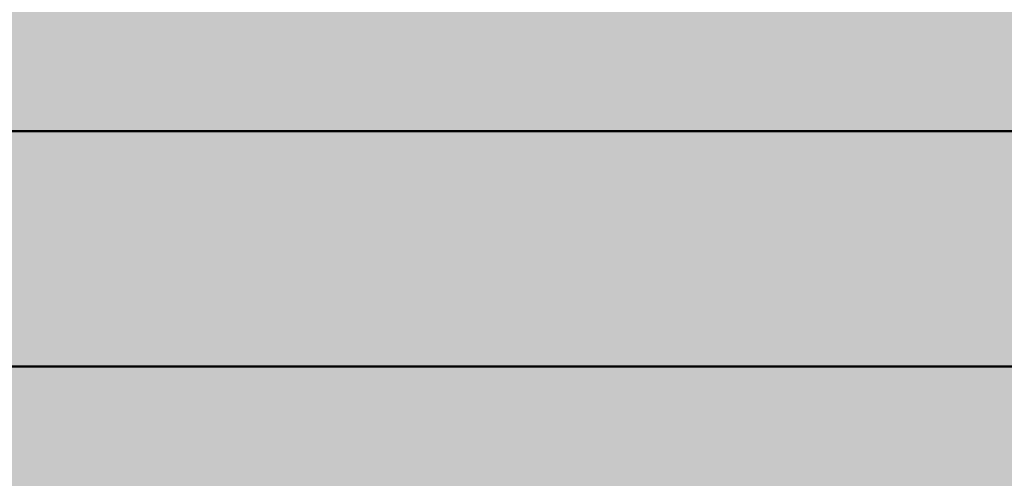
# Model space of a CAD drawing. Units: millimetres. Extents: x 0 to 2267, y 0 to 1823.
# Tile 138 of 256: x 1760 to 1802, y 1113 to 1132. Entities that reach past the tile are written whole.
import ezdxf

# ---------------------------------------------------------------- set-up
doc = ezdxf.new("R2010")
doc.units = ezdxf.units.MM
doc.header["$MEASUREMENT"] = 0
for name, color, linetype, lineweight in [('M-DIMS', 2, 'Continuous', 25), ('M-HATC', 252, 'Continuous', 18), ('M-OUTL', 7, 'Continuous', 50)]:
    doc.layers.add(name, color=color, linetype=linetype, lineweight=lineweight)
doc.styles.get("Standard").update_dxf_attribs({"font": 'arial.ttf'})
doc.dimstyles.get("Standard").update_dxf_attribs({"dimtxt": 7, "dimasz": 4, "dimexe": 0.18, "dimexo": 0.0625, "dimgap": 0.09, "dimtad": 0, "dimdec": 0, "dimzin": 0, "dimdsep": 46, "dimtxsty": 'Standard', "dimcen": 0.09, "dimadec": 0, "dimazin": 0, "dimtfac": 1, "dimtdec": 0, "dimtofl": 0, "dimtmove": 0, "dimatfit": 3, "dimfxl": 1, "dimtolj": 1, "dimtzin": 0, "dimarcsym": 0})

# ---------------------------------------------------------------- blocks, each defined once
blk = doc.blocks.new('*D1')
at = {"layer": 'Defpoints', "color": 0, "transparency": 16777216}
for p in [(1593.429, 1127.417), (1843.429, 1127.417), (1843.429, 955.628)]:
    blk.add_point(p, dxfattribs=at)
at = {"layer": 'M-DIMS', "color": 0, "lineweight": -2, "transparency": 16777216}
for p, q in [((1593.429, 1127.355), (1593.429, 955.448)), ((1843.429, 1127.355), (1843.429, 955.448)), ((1597.429, 955.628), (1710.558, 955.628)), ((1839.429, 955.628), (1726.3, 955.628))]:
    blk.add_line(p, q, dxfattribs=at)
at = {"layer": 'M-DIMS', "color": 0, "transparency": 16777216}
for points in [[(1597.429, 956.294), (1597.429, 954.961), (1593.429, 955.628)], [(1839.429, 956.294), (1839.429, 954.961), (1843.429, 955.628)]]:
    blk.add_solid(points, dxfattribs=at)
at = {"layer": 'M-DIMS', "color": 0, "transparency": 16777216, "insert": (1718.429, 955.628), "char_height": 7, "attachment_point": 5}
blk.add_mtext('\\A1;250', dxfattribs=at)

msp = doc.modelspace()

# ---------------------------------------------------------------- hatches: boundary and pattern name
at = {"layer": 'M-HATC'}
h = msp.add_hatch(color=256, dxfattribs=at)
h.dxf.hatch_style = 1
h.paths.add_polyline_path([(2065.771, 1618.062, 0.236068), (2055.771, 1638.062), (1381.087, 1638.062, 0.236068), (1371.087, 1618.062), (1371.087, 1603.062), (2055.771, 1603.062), (2065.771, 1603.062)])
h.paths.add_polyline_path([(2062.772, 1550.296), (2062.772, 1560.296), (1374.086, 1560.296), (1374.086, 1550.296), (1374.086, 1540.296), (1384.086, 1540.296), (1389.086, 1540.296), (2062.772, 1540.296)])
h.paths.add_polyline_path([(1930.929, 1282.766), (1505.929, 1282.766), (1587.628, 1235.597, 0.131652), (1600.128, 1232.247), (1836.73, 1232.247, 0.131652), (1849.23, 1235.597)])
h.paths.add_polyline_path([(1930.929, 1117.417), (1905.929, 1117.417), (1505.929, 1117.417), (1505.929, 1077.417), (1930.929, 1077.417)])
h = msp.add_hatch(color=256, dxfattribs=at)
h.dxf.hatch_style = 1
h.paths.add_polyline_path([(2055.771, 1603.062), (1381.087, 1603.062), (1381.087, 1598.062), (2055.771, 1598.062)])
h.paths.add_polyline_path([(2055.771, 1598.062), (1381.087, 1598.062), (1381.087, 1593.062), (2055.771, 1593.062)])
h.paths.add_polyline_path([(2051.307, 1536.761), (1385.55, 1536.761), (1385.55, 1526.761), (1387.55, 1526.761), (1388.537, 1525.053), (1385.332, 1521.233), (1385.332, 1521.223), (2050.254, 1522.749), (2048.321, 1525.053), (2049.307, 1526.761), (2051.307, 1526.761)])
edge = h.paths.add_edge_path()
edge.add_arc((1847.535, 1379.149), 135, 222.60306, 222.89085, ccw=False)
edge.add_line((1748.166, 1287.766), (1683.092, 1287.766))
edge.add_arc((1583.724, 1379.149), 135, 317.10915, 317.39694, ccw=False)
edge.add_arc((1678.969, 1290.671), 5, 222.8909, 317.1091, ccw=False)
edge.add_arc((1774.213, 1379.149), 135, 222.60306, 222.89085, ccw=False)
edge.add_line((1674.845, 1287.766), (1609.771, 1287.766))
edge.add_arc((1510.403, 1379.149), 135, 317.10915, 317.39694, ccw=False)
edge.add_arc((1605.647, 1290.671), 5, 222.8909, 317.1091, ccw=False)
edge.add_arc((1700.892, 1379.149), 135, 222.60306, 222.89085, ccw=False)
edge.add_line((1601.524, 1287.766), (1536.45, 1287.766))
edge.add_arc((1437.081, 1379.149), 135, 317.10915, 317.39694, ccw=False)
edge.add_arc((1532.326, 1290.671), 5, 222.8909, 317.1091, ccw=False)
edge.add_arc((1627.571, 1379.149), 135, 222.60306, 222.89085, ccw=False)
edge.add_line((1528.203, 1287.766), (1505.929, 1287.766))
edge.add_spline(control_points=[(1505.929, 1287.766), (1504.262, 1287.766), (1504.262, 1282.766), (1505.929, 1282.766)], knot_values=[0, 0, 0, 0, 5, 5, 5, 5], degree=3, periodic=0)
edge.add_line((1505.929, 1282.766), (1930.929, 1282.766))
edge.add_spline(control_points=[(1930.929, 1282.766), (1932.596, 1282.766), (1932.596, 1287.766), (1930.929, 1287.766)], knot_values=[0, 0, 0, 0, 5, 5, 5, 5], degree=3, periodic=0)
edge.add_line((1930.929, 1287.766), (1903.056, 1287.766))
edge.add_arc((1803.688, 1379.149), 135, 317.10915, 317.39694, ccw=False)
edge.add_arc((1898.932, 1290.671), 5, 222.8909, 317.1091, ccw=False)
edge.add_arc((1994.177, 1379.149), 135, 222.60306, 222.89085, ccw=False)
edge.add_line((1894.809, 1287.766), (1829.735, 1287.766))
edge.add_arc((1730.366, 1379.149), 135, 317.10915, 317.39694, ccw=False)
edge.add_arc((1825.611, 1290.671), 5, 222.8909, 317.1091, ccw=False)
edge.add_arc((1920.856, 1379.149), 135, 222.60306, 222.89085, ccw=False)
edge.add_line((1821.487, 1287.766), (1756.413, 1287.766))
edge.add_arc((1657.045, 1379.149), 135, 317.10915, 317.39694, ccw=False)
edge.add_arc((1752.29, 1290.671), 5, 222.8909, 317.1091, ccw=False)
edge = h.paths.add_edge_path()
edge.add_spline(control_points=[(1843.429, 1227.247), (1845.096, 1227.247), (1845.096, 1232.247), (1843.429, 1232.247)], knot_values=[0, 0, 0, 0, 5, 5, 5, 5], degree=3, periodic=0)
edge.add_line((1843.429, 1232.247), (1593.429, 1232.247))
edge.add_spline(control_points=[(1593.429, 1232.247), (1591.762, 1232.247), (1591.762, 1227.247), (1593.429, 1227.247)], knot_values=[0, 0, 0, 0, 5, 5, 5, 5], degree=3, periodic=0)
edge.add_line((1593.429, 1227.247), (1843.429, 1227.247))
h.paths.add_polyline_path([(1905.929, 1127.417), (1530.929, 1127.417, 0.414214), (1520.929, 1117.417), (1530.929, 1117.417), (1915.929, 1117.417, 0.414214)])
edge = h.paths.add_edge_path()
edge.add_arc((1397.086, 1498.408), 12.73, 90.7821, 190.8787, ccw=False)
edge.add_line((1396.912, 1511.136), (1428.01, 1511.349))
edge.add_line((1428.01, 1511.349), (1433.01, 1511.349))
edge.add_line((1433.01, 1511.349), (1434.439, 1511.349))
edge.add_arc((1419.474, 1498.08), 20, 41.561, 74.0821)
edge.add_line((1424.959, 1517.314), (1399.935, 1517.256))
edge.add_spline(control_points=[(1399.931, 1517.256), (1399.884, 1517.213), (1399.833, 1517.169), (1399.777, 1517.124)], knot_values=[11.567499, 11.567499, 11.567499, 11.567499, 11.814249, 11.814249, 11.814249, 11.814249], degree=3, periodic=0)
edge.add_spline(control_points=[(1399.633, 1517.01), (1399.583, 1516.972), (1399.531, 1516.934), (1399.476, 1516.895)], knot_values=[11.167718, 11.167718, 11.167718, 11.167718, 11.365188, 11.365188, 11.365188, 11.365188], degree=3, periodic=0)
edge.add_spline(control_points=[(1399.34, 1516.8), (1399.151, 1516.672), (1398.938, 1516.538), (1398.704, 1516.399)], knot_values=[10.376405, 10.376405, 10.376405, 10.376405, 11.00994, 11.00994, 11.00994, 11.00994], degree=3, periodic=0)
edge.add_spline(control_points=[(1398.657, 1516.372), (1398.579, 1516.326), (1398.498, 1516.28), (1398.415, 1516.233)], knot_values=[10.125175, 10.125175, 10.125175, 10.125175, 10.334406, 10.334406, 10.334406, 10.334406], degree=3, periodic=0)
edge.add_spline(control_points=[(1398.264, 1516.149), (1398.196, 1516.111), (1398.126, 1516.073), (1398.055, 1516.035)], knot_values=[9.832246, 9.832246, 9.832246, 9.832246, 9.999658, 9.999658, 9.999658, 9.999658], degree=3, periodic=0)
edge.add_spline(control_points=[(1397.999, 1516.005), (1397.731, 1515.862), (1397.446, 1515.717), (1397.147, 1515.571)], knot_values=[9.161808, 9.161808, 9.161808, 9.161808, 9.787769, 9.787769, 9.787769, 9.787769], degree=3, periodic=0)
edge.add_spline(control_points=[(1397.147, 1515.571), (1396.842, 1515.423), (1396.522, 1515.274), (1396.191, 1515.126)], knot_values=[8.524455, 8.524455, 8.524455, 8.524455, 9.161808, 9.161808, 9.161808, 9.161808], degree=3, periodic=0)
edge.add_spline(control_points=[(1396.078, 1515.076), (1395.985, 1515.035), (1395.892, 1514.994), (1395.798, 1514.953)], knot_values=[8.275193, 8.275193, 8.275193, 8.275193, 8.451726, 8.451726, 8.451726, 8.451726], degree=3, periodic=0)
edge.add_spline(control_points=[(1395.602, 1514.869), (1395.5, 1514.826), (1395.397, 1514.782), (1395.293, 1514.739)], knot_values=[7.962917, 7.962917, 7.962917, 7.962917, 8.152764, 8.152764, 8.152764, 8.152764], degree=3, periodic=0)
edge.add_spline(control_points=[(1395.212, 1514.706), (1394.828, 1514.547), (1394.435, 1514.393), (1394.036, 1514.244)], knot_values=[7.21254, 7.21254, 7.21254, 7.21254, 7.913148, 7.913148, 7.913148, 7.913148], degree=3, periodic=0)
edge.add_spline(control_points=[(1394.036, 1514.244), (1393.708, 1514.121), (1393.375, 1514.003), (1393.043, 1513.889)], knot_values=[6.633733, 6.633733, 6.633733, 6.633733, 7.21254, 7.21254, 7.21254, 7.21254], degree=3, periodic=0)
edge.add_spline(control_points=[(1392.821, 1513.815), (1392.72, 1513.781), (1392.618, 1513.748), (1392.517, 1513.715)], knot_values=[6.328796, 6.328796, 6.328796, 6.328796, 6.505493, 6.505493, 6.505493, 6.505493], degree=3, periodic=0)
edge.add_spline(control_points=[(1392.517, 1513.715), (1392.319, 1513.652), (1392.121, 1513.59), (1391.924, 1513.531)], knot_values=[5.984605, 5.984605, 5.984605, 5.984605, 6.328796, 6.328796, 6.328796, 6.328796], degree=3, periodic=0)
edge.add_spline(control_points=[(1391.792, 1513.491), (1391.312, 1513.35), (1390.838, 1513.224), (1390.378, 1513.117)], knot_values=[5.066697, 5.066697, 5.066697, 5.066697, 5.907055, 5.907055, 5.907055, 5.907055], degree=3, periodic=0)
edge.add_spline(control_points=[(1390.378, 1513.117), (1390.18, 1513.071), (1389.984, 1513.028), (1389.791, 1512.99)], knot_values=[4.70367, 4.70367, 4.70367, 4.70367, 5.066695, 5.066695, 5.066695, 5.066695], degree=3, periodic=0)
edge.add_spline(control_points=[(1389.422, 1512.92), (1389.246, 1512.889), (1389.073, 1512.862), (1388.904, 1512.838)], knot_values=[4.130571, 4.130571, 4.130571, 4.130571, 4.469816, 4.469816, 4.469816, 4.469816], degree=3, periodic=0)
edge.add_spline(control_points=[(1388.904, 1512.838), (1388.591, 1512.795), (1388.291, 1512.764), (1388.007, 1512.749)], knot_values=[3.504031, 3.504031, 3.504031, 3.504031, 4.130571, 4.130571, 4.130571, 4.130571], degree=3, periodic=0)
edge.add_spline(control_points=[(1387.936, 1512.746), (1387.854, 1512.742), (1387.773, 1512.74), (1387.694, 1512.739)], knot_values=[3.268866, 3.268866, 3.268866, 3.268866, 3.451164, 3.451164, 3.451164, 3.451164], degree=3, periodic=0)
edge.add_spline(control_points=[(1387.335, 1512.744), (1387.208, 1512.75), (1387.085, 1512.76), (1386.967, 1512.774)], knot_values=[2.670686, 2.670686, 2.670686, 2.670686, 2.984, 2.984, 2.984, 2.984], degree=3, periodic=0)
edge.add_spline(control_points=[(1386.833, 1512.792), (1386.821, 1512.794), (1386.809, 1512.796), (1386.797, 1512.798)], knot_values=[2.516981, 2.516981, 2.516981, 2.516981, 2.549528, 2.549528, 2.549528, 2.549528], degree=3, periodic=0)
edge.add_spline(control_points=[(1386.453, 1512.873), (1386.426, 1512.881), (1386.399, 1512.889), (1386.373, 1512.897)], knot_values=[2.095869, 2.095869, 2.095869, 2.095869, 2.17941, 2.17941, 2.17941, 2.17941], degree=3, periodic=0)
edge.add_spline(control_points=[(1386.069, 1513.019), (1386.063, 1513.022), (1386.058, 1513.025), (1386.052, 1513.028)], knot_values=[1.72453, 1.72453, 1.72453, 1.72453, 1.745933, 1.745933, 1.745933, 1.745933], degree=3, periodic=0)
edge.add_arc((1399.474, 1498.08), 20, 131.8243, 180)
edge.add_arc((1630.334, 1505.548), 250.971, 181.70518, 236.42798)
edge.add_arc((1605.34, 1483.304), 218.782, 238.66083, 243.34961)
edge.add_arc((1647.091, 1510.359), 262.899, 183.12984, 237.85344, ccw=False)
h.paths.add_polyline_path([(1406.537, 1391.964, 0.149382), (1491.551, 1296.442, -0.129517)], flags=17)
edge = h.paths.add_edge_path()
edge.add_arc((2037.384, 1498.08), 20, 0, 48.2659)
edge.add_spline(control_points=[(2050.697, 1513.005), (2050.651, 1512.985), (2050.603, 1512.966), (2050.554, 1512.948)], knot_values=[1.835652, 1.835652, 1.835652, 1.835652, 2.000781, 2.000781, 2.000781, 2.000781], degree=3, periodic=0)
edge.add_spline(control_points=[(2050.462, 1512.917), (2050.479, 1512.922), (2050.496, 1512.928), (2050.513, 1512.934)], knot_values=[2.045477, 2.045477, 2.045477, 2.045477, 2.101389, 2.101389, 2.101389, 2.101389], degree=3, periodic=0)
edge.add_spline(control_points=[(2050.129, 1512.834), (2050.198, 1512.847), (2050.266, 1512.862), (2050.331, 1512.879)], knot_values=[2.237629, 2.237629, 2.237629, 2.237629, 2.435841, 2.435841, 2.435841, 2.435841], degree=3, periodic=0)
edge.add_spline(control_points=[(2050.095, 1512.828), (2050.106, 1512.83), (2050.118, 1512.832), (2050.129, 1512.834)], knot_values=[2.435841, 2.435841, 2.435841, 2.435841, 2.468321, 2.468321, 2.468321, 2.468321], degree=3, periodic=0)
edge.add_spline(control_points=[(2049.784, 1512.785), (2049.855, 1512.792), (2049.924, 1512.801), (2049.992, 1512.811)], knot_values=[2.563852, 2.563852, 2.563852, 2.563852, 2.748541, 2.748541, 2.748541, 2.748541], degree=3, periodic=0)
edge.add_spline(control_points=[(2049.405, 1512.762), (2049.536, 1512.765), (2049.663, 1512.773), (2049.784, 1512.785)], knot_values=[2.748541, 2.748541, 2.748541, 2.748541, 3.064882, 3.064882, 3.064882, 3.064882], degree=3, periodic=0)
edge.add_spline(control_points=[(2049.17, 1512.76), (2049.234, 1512.759), (2049.297, 1512.759), (2049.358, 1512.761)], knot_values=[3.102309, 3.102309, 3.102309, 3.102309, 3.2503, 3.2503, 3.2503, 3.2503], degree=3, periodic=0)
edge.add_spline(control_points=[(2048.857, 1512.769), (2048.964, 1512.764), (2049.068, 1512.761), (2049.17, 1512.76)], knot_values=[3.2503, 3.2503, 3.2503, 3.2503, 3.486069, 3.486069, 3.486069, 3.486069], degree=3, periodic=0)
edge.add_spline(control_points=[(2048.692, 1512.779), (2048.373, 1512.801), (2048.035, 1512.841), (2047.682, 1512.897)], knot_values=[3.606429, 3.606429, 3.606429, 3.606429, 4.2989, 4.2989, 4.2989, 4.2989], degree=3, periodic=0)
edge.add_spline(control_points=[(2047.682, 1512.897), (2047.546, 1512.919), (2047.408, 1512.942), (2047.268, 1512.969)], knot_values=[4.2989, 4.2989, 4.2989, 4.2989, 4.565769, 4.565769, 4.565769, 4.565769], degree=3, periodic=0)
edge.add_spline(control_points=[(2047.268, 1512.969), (2047.145, 1512.991), (2047.021, 1513.016), (2046.895, 1513.042)], knot_values=[4.565769, 4.565769, 4.565769, 4.565769, 4.799971, 4.799971, 4.799971, 4.799971], degree=3, periodic=0)
edge.add_spline(control_points=[(2046.895, 1513.042), (2046.529, 1513.119), (2046.151, 1513.209), (2045.768, 1513.311)], knot_values=[4.799971, 4.799971, 4.799971, 4.799971, 5.483718, 5.483718, 5.483718, 5.483718], degree=3, periodic=0)
edge.add_spline(control_points=[(2045.768, 1513.311), (2045.372, 1513.415), (2044.97, 1513.532), (2044.566, 1513.659)], knot_values=[5.483718, 5.483718, 5.483718, 5.483718, 6.187866, 6.187866, 6.187866, 6.187866], degree=3, periodic=0)
edge.add_spline(control_points=[(2044.566, 1513.659), (2044.415, 1513.706), (2044.263, 1513.755), (2044.112, 1513.805)], knot_values=[6.187866, 6.187866, 6.187866, 6.187866, 6.451551, 6.451551, 6.451551, 6.451551], degree=3, periodic=0)
edge.add_spline(control_points=[(2044.112, 1513.805), (2043.997, 1513.843), (2043.882, 1513.881), (2043.767, 1513.92)], knot_values=[6.451551, 6.451551, 6.451551, 6.451551, 6.651434, 6.651434, 6.651434, 6.651434], degree=3, periodic=0)
edge.add_spline(control_points=[(2043.767, 1513.92), (2043.372, 1514.055), (2042.977, 1514.198), (2042.589, 1514.346)], knot_values=[6.651434, 6.651434, 6.651434, 6.651434, 7.338879, 7.338879, 7.338879, 7.338879], degree=3, periodic=0)
edge.add_spline(control_points=[(2042.589, 1514.346), (2042.164, 1514.507), (2041.746, 1514.675), (2041.341, 1514.846)], knot_values=[7.338879, 7.338879, 7.338879, 7.338879, 8.089209, 8.089209, 8.089209, 8.089209], degree=3, periodic=0)
edge.add_spline(control_points=[(2041.341, 1514.846), (2041.103, 1514.946), (2040.869, 1515.048), (2040.64, 1515.15)], knot_values=[8.089209, 8.089209, 8.089209, 8.089209, 8.529587, 8.529587, 8.529587, 8.529587], degree=3, periodic=0)
edge.add_spline(control_points=[(2040.51, 1515.209), (2040.082, 1515.402), (2039.675, 1515.597), (2039.295, 1515.789)], knot_values=[8.613818, 8.613818, 8.613818, 8.613818, 9.44571, 9.44571, 9.44571, 9.44571], degree=3, periodic=0)
edge.add_spline(control_points=[(2039.295, 1515.789), (2039.062, 1515.907), (2038.839, 1516.025), (2038.629, 1516.14)], knot_values=[9.44571, 9.44571, 9.44571, 9.44571, 9.956404, 9.956404, 9.956404, 9.956404], degree=3, periodic=0)
edge.add_spline(control_points=[(2038.629, 1516.14), (2038.519, 1516.2), (2038.412, 1516.26), (2038.309, 1516.319)], knot_values=[9.956404, 9.956404, 9.956404, 9.956404, 10.223542, 10.223542, 10.223542, 10.223542], degree=3, periodic=0)
edge.add_spline(control_points=[(2038.309, 1516.319), (2038.214, 1516.374), (2038.122, 1516.428), (2038.033, 1516.481)], knot_values=[10.223542, 10.223542, 10.223542, 10.223542, 10.47051, 10.47051, 10.47051, 10.47051], degree=3, periodic=0)
edge.add_spline(control_points=[(2038.033, 1516.481), (2037.786, 1516.63), (2037.564, 1516.773), (2037.372, 1516.909)], knot_values=[10.47051, 10.47051, 10.47051, 10.47051, 11.15767, 11.15767, 11.15767, 11.15767], degree=3, periodic=0)
edge.add_spline(control_points=[(2037.372, 1516.909), (2037.279, 1516.975), (2037.193, 1517.04), (2037.114, 1517.102)], knot_values=[11.15767, 11.15767, 11.15767, 11.15767, 11.49227, 11.49227, 11.49227, 11.49227], degree=3, periodic=0)
edge.add_spline(control_points=[(2036.856, 1517.326), (2036.915, 1517.269), (2036.981, 1517.21), (2037.056, 1517.149)], knot_values=[11.577341, 11.577341, 11.577341, 11.577341, 11.91035, 11.91035, 11.91035, 11.91035], degree=3, periodic=0)
edge.add_spline(control_points=[(2036.807, 1517.375), (2036.823, 1517.359), (2036.839, 1517.342), (2036.856, 1517.326)], knot_values=[11.91035, 11.91035, 11.91035, 11.91035, 12.007402, 12.007402, 12.007402, 12.007402], degree=3, periodic=0)
edge.add_spline(control_points=[(2036.702, 1517.494), (2036.71, 1517.483), (2036.72, 1517.472), (2036.729, 1517.461)], knot_values=[12.184155, 12.184155, 12.184155, 12.184155, 12.255409, 12.255409, 12.255409, 12.255409], degree=3, periodic=0)
edge.add_spline(control_points=[(2036.616, 1517.621), (2036.62, 1517.613), (2036.624, 1517.606), (2036.629, 1517.598)], knot_values=[12.487913, 12.487913, 12.487913, 12.487913, 12.541035, 12.541035, 12.541035, 12.541035], degree=3, periodic=0)
edge.add_spline(control_points=[(2036.563, 1517.786), (2036.564, 1517.779), (2036.564, 1517.773), (2036.565, 1517.766)], knot_values=[12.911761, 12.911761, 12.911761, 12.911761, 12.968286, 12.968286, 12.968286, 12.968286], degree=3, periodic=0)
edge.add_spline(control_points=[(2036.617, 1517.93), (2036.612, 1517.926), (2036.609, 1517.921), (2036.605, 1517.916)], knot_values=[13.382527, 13.382527, 13.382527, 13.382527, 13.433791, 13.433791, 13.433791, 13.433791], degree=3, periodic=0)
edge.add_spline(control_points=[(2036.749, 1518.017), (2036.736, 1518.012), (2036.724, 1518.006), (2036.712, 1518)], knot_values=[13.726299, 13.726299, 13.726299, 13.726299, 13.809928, 13.809928, 13.809928, 13.809928], degree=3, periodic=0)
edge.add_spline(control_points=[(2036.86, 1518.053), (2036.839, 1518.047), (2036.818, 1518.042), (2036.799, 1518.035)], knot_values=[13.910887, 13.910887, 13.910887, 13.910887, 14.02153, 14.02153, 14.02153, 14.02153], degree=3, periodic=0)
edge.add_line((2036.964, 1518.08), (2032.384, 1518.08))
edge.add_line((2032.384, 1518.08), (2027.384, 1518.08))
edge.add_line((2027.384, 1518.08), (2022.384, 1518.08))
edge.add_line((2022.384, 1518.08), (2017.384, 1518.08))
edge.add_arc((2017.384, 1498.08), 20, 90, 138.439)
edge.add_line((2002.419, 1511.349), (2003.848, 1511.349))
edge.add_line((2003.848, 1511.349), (2008.848, 1511.349))
edge.add_line((2008.848, 1511.349), (2039.772, 1511.138))
edge.add_arc((2039.772, 1498.408), 12.73, -10.8787, 90, ccw=False)
edge.add_arc((1789.767, 1510.359), 262.899, 302.14656, 356.87016, ccw=False)
edge.add_arc((1831.518, 1483.304), 218.782, 296.65039, 301.33917)
edge.add_arc((1806.524, 1505.548), 250.971, 303.57202, 358.29482)
h.paths.add_polyline_path([(2030.321, 1391.964, -0.129517), (1945.307, 1296.442, 0.149382)], flags=17)
edge = h.paths.add_edge_path()
edge.add_spline(control_points=[(2037.246, 1518.082), (2037.29, 1518.081), (2037.336, 1518.08), (2037.384, 1518.08)], knot_values=[0.000012, 0.000012, 0.000012, 0.000012, 0.144754, 0.144754, 0.144754, 0.144754], degree=3, periodic=0)
edge.add_line((2037.336, 1518.08), (2037.01, 1518.08))
edge.add_spline(control_points=[(2037.01, 1518.08), (2036.982, 1518.077), (2036.956, 1518.073), (2036.931, 1518.068)], knot_values=[14.13465, 14.13465, 14.13465, 14.13465, 14.247197, 14.247197, 14.247197, 14.247197], degree=3, periodic=0)
edge.add_spline(control_points=[(2036.931, 1518.068), (2036.928, 1518.067), (2036.924, 1518.067), (2036.921, 1518.066)], knot_values=[14.118315, 14.118315, 14.118315, 14.118315, 14.13465, 14.13465, 14.13465, 14.13465], degree=3, periodic=0)
edge.add_spline(control_points=[(2036.921, 1518.066), (2036.912, 1518.064), (2036.903, 1518.063), (2036.895, 1518.061)], knot_values=[14.078086, 14.078086, 14.078086, 14.078086, 14.118315, 14.118315, 14.118315, 14.118315], degree=3, periodic=0)
edge.add_spline(control_points=[(2036.895, 1518.061), (2036.883, 1518.058), (2036.872, 1518.056), (2036.86, 1518.053)], knot_values=[14.02153, 14.02153, 14.02153, 14.02153, 14.078086, 14.078086, 14.078086, 14.078086], degree=3, periodic=0)
edge.add_spline(control_points=[(2036.86, 1518.053), (2036.839, 1518.047), (2036.818, 1518.042), (2036.799, 1518.035)], knot_values=[13.910887, 13.910887, 13.910887, 13.910887, 14.02153, 14.02153, 14.02153, 14.02153], degree=3, periodic=0)
edge.add_spline(control_points=[(2036.799, 1518.035), (2036.798, 1518.035), (2036.797, 1518.035), (2036.797, 1518.035)], knot_values=[13.906906, 13.906906, 13.906906, 13.906906, 13.910887, 13.910887, 13.910887, 13.910887], degree=3, periodic=0)
edge.add_spline(control_points=[(2036.797, 1518.035), (2036.788, 1518.032), (2036.78, 1518.029), (2036.772, 1518.026)], knot_values=[13.857826, 13.857826, 13.857826, 13.857826, 13.906906, 13.906906, 13.906906, 13.906906], degree=3, periodic=0)
edge.add_spline(control_points=[(2036.772, 1518.026), (2036.764, 1518.023), (2036.756, 1518.02), (2036.749, 1518.017)], knot_values=[13.809928, 13.809928, 13.809928, 13.809928, 13.857826, 13.857826, 13.857826, 13.857826], degree=3, periodic=0)
edge.add_spline(control_points=[(2036.749, 1518.017), (2036.736, 1518.012), (2036.724, 1518.006), (2036.712, 1518)], knot_values=[13.726299, 13.726299, 13.726299, 13.726299, 13.809928, 13.809928, 13.809928, 13.809928], degree=3, periodic=0)
edge.add_spline(control_points=[(2036.712, 1518), (2036.712, 1518), (2036.712, 1518), (2036.711, 1518)], knot_values=[13.723993, 13.723993, 13.723993, 13.723993, 13.726299, 13.726299, 13.726299, 13.726299], degree=3, periodic=0)
edge.add_spline(control_points=[(2036.711, 1518), (2036.706, 1517.997), (2036.701, 1517.994), (2036.696, 1517.992)], knot_values=[13.686536, 13.686536, 13.686536, 13.686536, 13.723993, 13.723993, 13.723993, 13.723993], degree=3, periodic=0)
edge.add_spline(control_points=[(2036.696, 1517.992), (2036.692, 1517.989), (2036.687, 1517.987), (2036.683, 1517.984)], knot_values=[13.651251, 13.651251, 13.651251, 13.651251, 13.686536, 13.686536, 13.686536, 13.686536], degree=3, periodic=0)
edge.add_spline(control_points=[(2036.683, 1517.984), (2036.676, 1517.98), (2036.67, 1517.976), (2036.664, 1517.971)], knot_values=[13.596804, 13.596804, 13.596804, 13.596804, 13.651251, 13.651251, 13.651251, 13.651251], degree=3, periodic=0)
edge.add_spline(control_points=[(2036.664, 1517.971), (2036.664, 1517.971), (2036.663, 1517.971), (2036.663, 1517.971)], knot_values=[13.593956, 13.593956, 13.593956, 13.593956, 13.596804, 13.596804, 13.596804, 13.596804], degree=3, periodic=0)
edge.add_spline(control_points=[(2036.663, 1517.971), (2036.66, 1517.969), (2036.658, 1517.967), (2036.655, 1517.965)], knot_values=[13.570322, 13.570322, 13.570322, 13.570322, 13.593956, 13.593956, 13.593956, 13.593956], degree=3, periodic=0)
edge.add_spline(control_points=[(2036.655, 1517.965), (2036.653, 1517.963), (2036.65, 1517.961), (2036.647, 1517.959)], knot_values=[13.545477, 13.545477, 13.545477, 13.545477, 13.570322, 13.570322, 13.570322, 13.570322], degree=3, periodic=0)
edge.add_spline(control_points=[(2036.647, 1517.959), (2036.647, 1517.959), (2036.647, 1517.959), (2036.647, 1517.959)], knot_values=[13.543931, 13.543931, 13.543931, 13.543931, 13.545477, 13.545477, 13.545477, 13.545477], degree=3, periodic=0)
edge.add_spline(control_points=[(2036.647, 1517.959), (2036.641, 1517.954), (2036.636, 1517.949), (2036.631, 1517.945)], knot_values=[13.488237, 13.488237, 13.488237, 13.488237, 13.543931, 13.543931, 13.543931, 13.543931], degree=3, periodic=0)
edge.add_spline(control_points=[(2036.631, 1517.945), (2036.628, 1517.942), (2036.626, 1517.94), (2036.623, 1517.937)], knot_values=[13.460307, 13.460307, 13.460307, 13.460307, 13.488237, 13.488237, 13.488237, 13.488237], degree=3, periodic=0)
edge.add_spline(control_points=[(2036.623, 1517.937), (2036.622, 1517.936), (2036.62, 1517.934), (2036.618, 1517.932)], knot_values=[13.439712, 13.439712, 13.439712, 13.439712, 13.460307, 13.460307, 13.460307, 13.460307], degree=3, periodic=0)
edge.add_spline(control_points=[(2036.618, 1517.932), (2036.618, 1517.931), (2036.617, 1517.931), (2036.617, 1517.93)], knot_values=[13.433791, 13.433791, 13.433791, 13.433791, 13.439712, 13.439712, 13.439712, 13.439712], degree=3, periodic=0)
edge.add_spline(control_points=[(2036.617, 1517.93), (2036.612, 1517.926), (2036.609, 1517.921), (2036.605, 1517.916)], knot_values=[13.382527, 13.382527, 13.382527, 13.382527, 13.433791, 13.433791, 13.433791, 13.433791], degree=3, periodic=0)
edge.add_spline(control_points=[(2036.605, 1517.916), (2036.603, 1517.913), (2036.6, 1517.91), (2036.598, 1517.907)], knot_values=[13.350017, 13.350017, 13.350017, 13.350017, 13.382527, 13.382527, 13.382527, 13.382527], degree=3, periodic=0)
edge.add_spline(control_points=[(2036.598, 1517.907), (2036.597, 1517.906), (2036.596, 1517.904), (2036.595, 1517.903)], knot_values=[13.333922, 13.333922, 13.333922, 13.333922, 13.350017, 13.350017, 13.350017, 13.350017], degree=3, periodic=0)
edge.add_spline(control_points=[(2036.595, 1517.903), (2036.595, 1517.902), (2036.594, 1517.901), (2036.593, 1517.9)], knot_values=[13.323828, 13.323828, 13.323828, 13.323828, 13.333922, 13.333922, 13.333922, 13.333922], degree=3, periodic=0)
edge.add_spline(control_points=[(2036.593, 1517.9), (2036.59, 1517.895), (2036.588, 1517.891), (2036.585, 1517.886)], knot_values=[13.277545, 13.277545, 13.277545, 13.277545, 13.323828, 13.323828, 13.323828, 13.323828], degree=3, periodic=0)
edge.add_spline(control_points=[(2036.585, 1517.886), (2036.584, 1517.883), (2036.582, 1517.879), (2036.58, 1517.875)], knot_values=[13.240119, 13.240119, 13.240119, 13.240119, 13.277545, 13.277545, 13.277545, 13.277545], degree=3, periodic=0)
edge.add_spline(control_points=[(2036.58, 1517.875), (2036.58, 1517.874), (2036.579, 1517.873), (2036.578, 1517.872)], knot_values=[13.228211, 13.228211, 13.228211, 13.228211, 13.240119, 13.240119, 13.240119, 13.240119], degree=3, periodic=0)
edge.add_spline(control_points=[(2036.578, 1517.872), (2036.578, 1517.87), (2036.577, 1517.869), (2036.577, 1517.868)], knot_values=[13.215717, 13.215717, 13.215717, 13.215717, 13.228211, 13.228211, 13.228211, 13.228211], degree=3, periodic=0)
edge.add_spline(control_points=[(2036.577, 1517.868), (2036.575, 1517.864), (2036.574, 1517.86), (2036.573, 1517.857)], knot_values=[13.179847, 13.179847, 13.179847, 13.179847, 13.215717, 13.215717, 13.215717, 13.215717], degree=3, periodic=0)
edge.add_spline(control_points=[(2036.573, 1517.857), (2036.571, 1517.851), (2036.57, 1517.846), (2036.569, 1517.841)], knot_values=[13.132017, 13.132017, 13.132017, 13.132017, 13.179847, 13.179847, 13.179847, 13.179847], degree=3, periodic=0)
edge.add_spline(control_points=[(2036.569, 1517.841), (2036.568, 1517.84), (2036.568, 1517.839), (2036.568, 1517.838)], knot_values=[13.122482, 13.122482, 13.122482, 13.122482, 13.132017, 13.132017, 13.132017, 13.132017], degree=3, periodic=0)
edge.add_spline(control_points=[(2036.568, 1517.838), (2036.568, 1517.836), (2036.567, 1517.835), (2036.567, 1517.833)], knot_values=[13.105592, 13.105592, 13.105592, 13.105592, 13.122482, 13.122482, 13.122482, 13.122482], degree=3, periodic=0)
edge.add_spline(control_points=[(2036.567, 1517.833), (2036.566, 1517.829), (2036.566, 1517.826), (2036.565, 1517.822)], knot_values=[13.074063, 13.074063, 13.074063, 13.074063, 13.105592, 13.105592, 13.105592, 13.105592], degree=3, periodic=0)
edge.add_spline(control_points=[(2036.565, 1517.822), (2036.565, 1517.822), (2036.565, 1517.822), (2036.565, 1517.822)], knot_values=[13.074043, 13.074043, 13.074043, 13.074043, 13.074063, 13.074063, 13.074063, 13.074063], degree=3, periodic=0)
edge.add_spline(control_points=[(2036.565, 1517.822), (2036.564, 1517.816), (2036.564, 1517.811), (2036.564, 1517.805)], knot_values=[13.021884, 13.021884, 13.021884, 13.021884, 13.074043, 13.074043, 13.074043, 13.074043], degree=3, periodic=0)
edge.add_spline(control_points=[(2036.564, 1517.805), (2036.564, 1517.804), (2036.564, 1517.803), (2036.564, 1517.803)], knot_values=[13.01674, 13.01674, 13.01674, 13.01674, 13.021884, 13.021884, 13.021884, 13.021884], degree=3, periodic=0)
edge.add_spline(control_points=[(2036.564, 1517.803), (2036.563, 1517.801), (2036.563, 1517.798), (2036.563, 1517.796)], knot_values=[12.996438, 12.996438, 12.996438, 12.996438, 13.01674, 13.01674, 13.01674, 13.01674], degree=3, periodic=0)
edge.add_spline(control_points=[(2036.563, 1517.796), (2036.563, 1517.793), (2036.563, 1517.789), (2036.563, 1517.786)], knot_values=[12.968286, 12.968286, 12.968286, 12.968286, 12.996438, 12.996438, 12.996438, 12.996438], degree=3, periodic=0)
edge.add_spline(control_points=[(2036.563, 1517.786), (2036.564, 1517.779), (2036.564, 1517.773), (2036.565, 1517.766)], knot_values=[12.911761, 12.911761, 12.911761, 12.911761, 12.968286, 12.968286, 12.968286, 12.968286], degree=3, periodic=0)
edge.add_spline(control_points=[(2036.565, 1517.766), (2036.565, 1517.766), (2036.565, 1517.766), (2036.565, 1517.766)], knot_values=[12.911017, 12.911017, 12.911017, 12.911017, 12.911761, 12.911761, 12.911761, 12.911761], degree=3, periodic=0)
edge.add_spline(control_points=[(2036.565, 1517.766), (2036.565, 1517.762), (2036.566, 1517.759), (2036.566, 1517.756)], knot_values=[12.88528, 12.88528, 12.88528, 12.88528, 12.911017, 12.911017, 12.911017, 12.911017], degree=3, periodic=0)
edge.add_spline(control_points=[(2036.566, 1517.756), (2036.567, 1517.753), (2036.567, 1517.751), (2036.568, 1517.748)], knot_values=[12.862519, 12.862519, 12.862519, 12.862519, 12.88528, 12.88528, 12.88528, 12.88528], degree=3, periodic=0)
edge.add_spline(control_points=[(2036.568, 1517.748), (2036.568, 1517.747), (2036.568, 1517.747), (2036.568, 1517.746)], knot_values=[12.858885, 12.858885, 12.858885, 12.858885, 12.862519, 12.862519, 12.862519, 12.862519], degree=3, periodic=0)
edge.add_spline(control_points=[(2036.568, 1517.746), (2036.569, 1517.74), (2036.571, 1517.733), (2036.572, 1517.726)], knot_values=[12.8053, 12.8053, 12.8053, 12.8053, 12.858885, 12.858885, 12.858885, 12.858885], degree=3, periodic=0)
edge.add_spline(control_points=[(2036.572, 1517.726), (2036.573, 1517.723), (2036.574, 1517.719), (2036.576, 1517.715)], knot_values=[12.775176, 12.775176, 12.775176, 12.775176, 12.8053, 12.8053, 12.8053, 12.8053], degree=3, periodic=0)
edge.add_spline(control_points=[(2036.576, 1517.715), (2036.576, 1517.713), (2036.577, 1517.71), (2036.578, 1517.708)], knot_values=[12.756759, 12.756759, 12.756759, 12.756759, 12.775176, 12.775176, 12.775176, 12.775176], degree=3, periodic=0)
edge.add_spline(control_points=[(2036.578, 1517.708), (2036.578, 1517.707), (2036.578, 1517.706), (2036.579, 1517.705)], knot_values=[12.748742, 12.748742, 12.748742, 12.748742, 12.756759, 12.756759, 12.756759, 12.756759], degree=3, periodic=0)
edge.add_spline(control_points=[(2036.579, 1517.705), (2036.581, 1517.698), (2036.583, 1517.692), (2036.586, 1517.685)], knot_values=[12.69959, 12.69959, 12.69959, 12.69959, 12.748742, 12.748742, 12.748742, 12.748742], degree=3, periodic=0)
edge.add_spline(control_points=[(2036.586, 1517.685), (2036.588, 1517.68), (2036.59, 1517.675), (2036.592, 1517.669)], knot_values=[12.659038, 12.659038, 12.659038, 12.659038, 12.69959, 12.69959, 12.69959, 12.69959], degree=3, periodic=0)
edge.add_spline(control_points=[(2036.592, 1517.669), (2036.594, 1517.665), (2036.596, 1517.66), (2036.598, 1517.656)], knot_values=[12.626806, 12.626806, 12.626806, 12.626806, 12.659038, 12.659038, 12.659038, 12.659038], degree=3, periodic=0)
edge.add_spline(control_points=[(2036.598, 1517.656), (2036.598, 1517.655), (2036.599, 1517.654), (2036.599, 1517.653)], knot_values=[12.619394, 12.619394, 12.619394, 12.619394, 12.626806, 12.626806, 12.626806, 12.626806], degree=3, periodic=0)
edge.add_spline(control_points=[(2036.599, 1517.653), (2036.604, 1517.642), (2036.61, 1517.632), (2036.616, 1517.621)], knot_values=[12.541039, 12.541039, 12.541039, 12.541039, 12.619394, 12.619394, 12.619394, 12.619394], degree=3, periodic=0)
edge.add_spline(control_points=[(2036.616, 1517.621), (2036.616, 1517.621), (2036.616, 1517.621), (2036.616, 1517.621)], knot_values=[12.541035, 12.541035, 12.541035, 12.541035, 12.541039, 12.541039, 12.541039, 12.541039], degree=3, periodic=0)
edge.add_spline(control_points=[(2036.616, 1517.621), (2036.62, 1517.613), (2036.624, 1517.606), (2036.629, 1517.598)], knot_values=[12.487913, 12.487913, 12.487913, 12.487913, 12.541035, 12.541035, 12.541035, 12.541035], degree=3, periodic=0)
edge.add_spline(control_points=[(2036.629, 1517.598), (2036.633, 1517.592), (2036.637, 1517.585), (2036.641, 1517.579)], knot_values=[12.443982, 12.443982, 12.443982, 12.443982, 12.487913, 12.487913, 12.487913, 12.487913], degree=3, periodic=0)
edge.add_spline(control_points=[(2036.641, 1517.579), (2036.641, 1517.578), (2036.642, 1517.576), (2036.643, 1517.575)], knot_values=[12.434996, 12.434996, 12.434996, 12.434996, 12.443982, 12.443982, 12.443982, 12.443982], degree=3, periodic=0)
edge.add_spline(control_points=[(2036.643, 1517.575), (2036.653, 1517.56), (2036.664, 1517.544), (2036.676, 1517.528)], knot_values=[12.329647, 12.329647, 12.329647, 12.329647, 12.434996, 12.434996, 12.434996, 12.434996], degree=3, periodic=0)
edge.add_spline(control_points=[(2036.676, 1517.528), (2036.684, 1517.517), (2036.693, 1517.505), (2036.702, 1517.494)], knot_values=[12.255409, 12.255409, 12.255409, 12.255409, 12.329647, 12.329647, 12.329647, 12.329647], degree=3, periodic=0)
edge.add_spline(control_points=[(2036.702, 1517.494), (2036.71, 1517.483), (2036.72, 1517.472), (2036.729, 1517.461)], knot_values=[12.184155, 12.184155, 12.184155, 12.184155, 12.255409, 12.255409, 12.255409, 12.255409], degree=3, periodic=0)
edge.add_spline(control_points=[(2036.729, 1517.461), (2036.744, 1517.444), (2036.759, 1517.426), (2036.775, 1517.409)], knot_values=[12.075961, 12.075961, 12.075961, 12.075961, 12.184155, 12.184155, 12.184155, 12.184155], degree=3, periodic=0)
edge.add_spline(control_points=[(2036.775, 1517.409), (2036.776, 1517.407), (2036.777, 1517.406), (2036.778, 1517.405)], knot_values=[12.069502, 12.069502, 12.069502, 12.069502, 12.075961, 12.075961, 12.075961, 12.075961], degree=3, periodic=0)
edge.add_spline(control_points=[(2036.778, 1517.405), (2036.788, 1517.395), (2036.797, 1517.385), (2036.807, 1517.375)], knot_values=[12.007402, 12.007402, 12.007402, 12.007402, 12.069502, 12.069502, 12.069502, 12.069502], degree=3, periodic=0)
edge.add_spline(control_points=[(2036.807, 1517.375), (2036.823, 1517.359), (2036.839, 1517.342), (2036.856, 1517.326)], knot_values=[11.91035, 11.91035, 11.91035, 11.91035, 12.007402, 12.007402, 12.007402, 12.007402], degree=3, periodic=0)
edge.add_spline(control_points=[(2036.856, 1517.326), (2036.915, 1517.269), (2036.981, 1517.21), (2037.056, 1517.149)], knot_values=[11.577341, 11.577341, 11.577341, 11.577341, 11.91035, 11.91035, 11.91035, 11.91035], degree=3, periodic=0)
edge.add_spline(control_points=[(2037.056, 1517.149), (2037.075, 1517.134), (2037.094, 1517.118), (2037.114, 1517.102)], knot_values=[11.49227, 11.49227, 11.49227, 11.49227, 11.577341, 11.577341, 11.577341, 11.577341], degree=3, periodic=0)
edge.add_spline(control_points=[(2037.114, 1517.102), (2037.193, 1517.04), (2037.279, 1516.975), (2037.372, 1516.909)], knot_values=[11.15767, 11.15767, 11.15767, 11.15767, 11.49227, 11.49227, 11.49227, 11.49227], degree=3, periodic=0)
edge.add_spline(control_points=[(2037.372, 1516.909), (2037.564, 1516.773), (2037.786, 1516.63), (2038.033, 1516.481)], knot_values=[10.47051, 10.47051, 10.47051, 10.47051, 11.15767, 11.15767, 11.15767, 11.15767], degree=3, periodic=0)
edge.add_spline(control_points=[(2038.033, 1516.481), (2038.122, 1516.428), (2038.214, 1516.374), (2038.309, 1516.319)], knot_values=[10.223542, 10.223542, 10.223542, 10.223542, 10.47051, 10.47051, 10.47051, 10.47051], degree=3, periodic=0)
edge.add_spline(control_points=[(2038.309, 1516.319), (2038.412, 1516.26), (2038.519, 1516.2), (2038.629, 1516.14)], knot_values=[9.956404, 9.956404, 9.956404, 9.956404, 10.223542, 10.223542, 10.223542, 10.223542], degree=3, periodic=0)
edge.add_spline(control_points=[(2038.629, 1516.14), (2038.839, 1516.025), (2039.062, 1515.907), (2039.295, 1515.789)], knot_values=[9.44571, 9.44571, 9.44571, 9.44571, 9.956404, 9.956404, 9.956404, 9.956404], degree=3, periodic=0)
edge.add_spline(control_points=[(2039.295, 1515.789), (2039.675, 1515.597), (2040.082, 1515.402), (2040.51, 1515.209)], knot_values=[8.613818, 8.613818, 8.613818, 8.613818, 9.44571, 9.44571, 9.44571, 9.44571], degree=3, periodic=0)
edge.add_spline(control_points=[(2040.51, 1515.209), (2040.553, 1515.189), (2040.597, 1515.17), (2040.64, 1515.15)], knot_values=[8.529587, 8.529587, 8.529587, 8.529587, 8.613818, 8.613818, 8.613818, 8.613818], degree=3, periodic=0)
edge.add_spline(control_points=[(2040.64, 1515.15), (2040.869, 1515.048), (2041.103, 1514.946), (2041.341, 1514.846)], knot_values=[8.089209, 8.089209, 8.089209, 8.089209, 8.529587, 8.529587, 8.529587, 8.529587], degree=3, periodic=0)
edge.add_spline(control_points=[(2041.341, 1514.846), (2041.746, 1514.675), (2042.164, 1514.507), (2042.589, 1514.346)], knot_values=[7.338879, 7.338879, 7.338879, 7.338879, 8.089209, 8.089209, 8.089209, 8.089209], degree=3, periodic=0)
edge.add_spline(control_points=[(2042.589, 1514.346), (2042.977, 1514.198), (2043.372, 1514.055), (2043.767, 1513.92)], knot_values=[6.651434, 6.651434, 6.651434, 6.651434, 7.338879, 7.338879, 7.338879, 7.338879], degree=3, periodic=0)
edge.add_spline(control_points=[(2043.767, 1513.92), (2043.882, 1513.881), (2043.997, 1513.843), (2044.112, 1513.805)], knot_values=[6.451551, 6.451551, 6.451551, 6.451551, 6.651434, 6.651434, 6.651434, 6.651434], degree=3, periodic=0)
edge.add_spline(control_points=[(2044.112, 1513.805), (2044.263, 1513.755), (2044.415, 1513.706), (2044.566, 1513.659)], knot_values=[6.187866, 6.187866, 6.187866, 6.187866, 6.451551, 6.451551, 6.451551, 6.451551], degree=3, periodic=0)
edge.add_spline(control_points=[(2044.566, 1513.659), (2044.97, 1513.532), (2045.372, 1513.415), (2045.768, 1513.311)], knot_values=[5.483718, 5.483718, 5.483718, 5.483718, 6.187866, 6.187866, 6.187866, 6.187866], degree=3, periodic=0)
edge.add_spline(control_points=[(2045.768, 1513.311), (2046.151, 1513.209), (2046.529, 1513.119), (2046.895, 1513.042)], knot_values=[4.799971, 4.799971, 4.799971, 4.799971, 5.483718, 5.483718, 5.483718, 5.483718], degree=3, periodic=0)
edge.add_spline(control_points=[(2046.895, 1513.042), (2047.021, 1513.016), (2047.145, 1512.991), (2047.268, 1512.969)], knot_values=[4.565769, 4.565769, 4.565769, 4.565769, 4.799971, 4.799971, 4.799971, 4.799971], degree=3, periodic=0)
edge.add_spline(control_points=[(2047.268, 1512.969), (2047.408, 1512.942), (2047.546, 1512.919), (2047.682, 1512.897)], knot_values=[4.2989, 4.2989, 4.2989, 4.2989, 4.565769, 4.565769, 4.565769, 4.565769], degree=3, periodic=0)
edge.add_spline(control_points=[(2047.682, 1512.897), (2048.035, 1512.841), (2048.373, 1512.801), (2048.692, 1512.779)], knot_values=[3.606429, 3.606429, 3.606429, 3.606429, 4.2989, 4.2989, 4.2989, 4.2989], degree=3, periodic=0)
edge.add_spline(control_points=[(2048.692, 1512.779), (2048.748, 1512.775), (2048.803, 1512.772), (2048.857, 1512.769)], knot_values=[3.486069, 3.486069, 3.486069, 3.486069, 3.606429, 3.606429, 3.606429, 3.606429], degree=3, periodic=0)
edge.add_spline(control_points=[(2048.857, 1512.769), (2048.964, 1512.764), (2049.068, 1512.761), (2049.17, 1512.76)], knot_values=[3.2503, 3.2503, 3.2503, 3.2503, 3.486069, 3.486069, 3.486069, 3.486069], degree=3, periodic=0)
edge.add_spline(control_points=[(2049.17, 1512.76), (2049.234, 1512.759), (2049.297, 1512.759), (2049.358, 1512.761)], knot_values=[3.102309, 3.102309, 3.102309, 3.102309, 3.2503, 3.2503, 3.2503, 3.2503], degree=3, periodic=0)
edge.add_spline(control_points=[(2049.358, 1512.761), (2049.374, 1512.761), (2049.39, 1512.761), (2049.405, 1512.762)], knot_values=[3.064882, 3.064882, 3.064882, 3.064882, 3.102309, 3.102309, 3.102309, 3.102309], degree=3, periodic=0)
edge.add_spline(control_points=[(2049.405, 1512.762), (2049.536, 1512.765), (2049.663, 1512.773), (2049.784, 1512.785)], knot_values=[2.748541, 2.748541, 2.748541, 2.748541, 3.064882, 3.064882, 3.064882, 3.064882], degree=3, periodic=0)
edge.add_spline(control_points=[(2049.784, 1512.785), (2049.855, 1512.792), (2049.924, 1512.801), (2049.992, 1512.811)], knot_values=[2.563852, 2.563852, 2.563852, 2.563852, 2.748541, 2.748541, 2.748541, 2.748541], degree=3, periodic=0)
edge.add_spline(control_points=[(2049.992, 1512.811), (2050.026, 1512.816), (2050.061, 1512.822), (2050.095, 1512.828)], knot_values=[2.468321, 2.468321, 2.468321, 2.468321, 2.563852, 2.563852, 2.563852, 2.563852], degree=3, periodic=0)
edge.add_spline(control_points=[(2050.095, 1512.828), (2050.106, 1512.83), (2050.118, 1512.832), (2050.129, 1512.834)], knot_values=[2.435841, 2.435841, 2.435841, 2.435841, 2.468321, 2.468321, 2.468321, 2.468321], degree=3, periodic=0)
edge.add_spline(control_points=[(2050.129, 1512.834), (2050.198, 1512.847), (2050.266, 1512.862), (2050.331, 1512.879)], knot_values=[2.237629, 2.237629, 2.237629, 2.237629, 2.435841, 2.435841, 2.435841, 2.435841], degree=3, periodic=0)
edge.add_spline(control_points=[(2050.331, 1512.879), (2050.375, 1512.891), (2050.419, 1512.903), (2050.462, 1512.917)], knot_values=[2.101389, 2.101389, 2.101389, 2.101389, 2.237629, 2.237629, 2.237629, 2.237629], degree=3, periodic=0)
edge.add_spline(control_points=[(2050.462, 1512.917), (2050.479, 1512.922), (2050.496, 1512.928), (2050.513, 1512.934)], knot_values=[2.045477, 2.045477, 2.045477, 2.045477, 2.101389, 2.101389, 2.101389, 2.101389], degree=3, periodic=0)
edge.add_spline(control_points=[(2050.513, 1512.934), (2050.527, 1512.938), (2050.54, 1512.943), (2050.554, 1512.948)], knot_values=[2.000781, 2.000781, 2.000781, 2.000781, 2.045477, 2.045477, 2.045477, 2.045477], degree=3, periodic=0)
edge.add_spline(control_points=[(2050.554, 1512.948), (2050.603, 1512.966), (2050.651, 1512.985), (2050.697, 1513.005)], knot_values=[1.835652, 1.835652, 1.835652, 1.835652, 2.000781, 2.000781, 2.000781, 2.000781], degree=3, periodic=0)
edge.add_arc((2037.384, 1498.08), 20, 48.2659, 90.1299)
edge = h.paths.add_edge_path(flags=16)
edge.add_spline(control_points=[(1386.139, 1512.986), (1388.92, 1511.739), (1398.039, 1515.519), (1399.931, 1517.256)], knot_values=[1.831046, 1.831046, 1.831046, 1.831046, 11.814249, 11.814249, 11.814249, 11.814249], degree=3, periodic=0)
edge.add_line((1399.931, 1517.256), (1393.743, 1517.242))
edge.add_arc((1399.474, 1498.08), 20, 106.6501, 131.8173)
h = msp.add_hatch(color=256, dxfattribs=at)
h.dxf.hatch_style = 1
h.paths.add_polyline_path([(2042.889, 1580.18), (2055.771, 1593.062), (1381.087, 1593.062), (1393.969, 1580.18), (1374.086, 1560.296), (2062.772, 1560.296)])
h.paths.add_polyline_path([(1843.429, 1201.33), (1843.429, 1227.247), (1593.429, 1227.247), (1593.429, 1201.33, -0.228274), (1574.599, 1162.235), (1530.929, 1127.417), (1905.929, 1127.417), (1862.259, 1162.235, -0.228274)])

# ---------------------------------------------------------------- linework, layer by layer
at = {"layer": 'M-OUTL'}
for p, q in [((1530.929, 1127.417), (1905.929, 1127.417)), ((1505.929, 1117.417), (1930.929, 1117.417)), ((1718.429, 1117.417), (1843.429, 1117.417))]:
    msp.add_line(p, q, dxfattribs=at)

# ---------------------------------------------------------------- dimensions: what is measured, and where the dimension line sits
at = {"layer": 'M-DIMS'}
dim = msp.add_linear_dim(base=(1843.429, 955.628), p1=(1593.429, 1127.417), p2=(1843.429, 1127.417), dimstyle='Standard', override={"dimclrd": 0, "dimclre": 0, "dimclrt": 0}, dxfattribs=at)
dim.commit()
dim.dimension.update_dxf_attribs({"geometry": '*D1', "text_midpoint": (1718.429, 955.628)})

doc.saveas('drawing.dxf')
